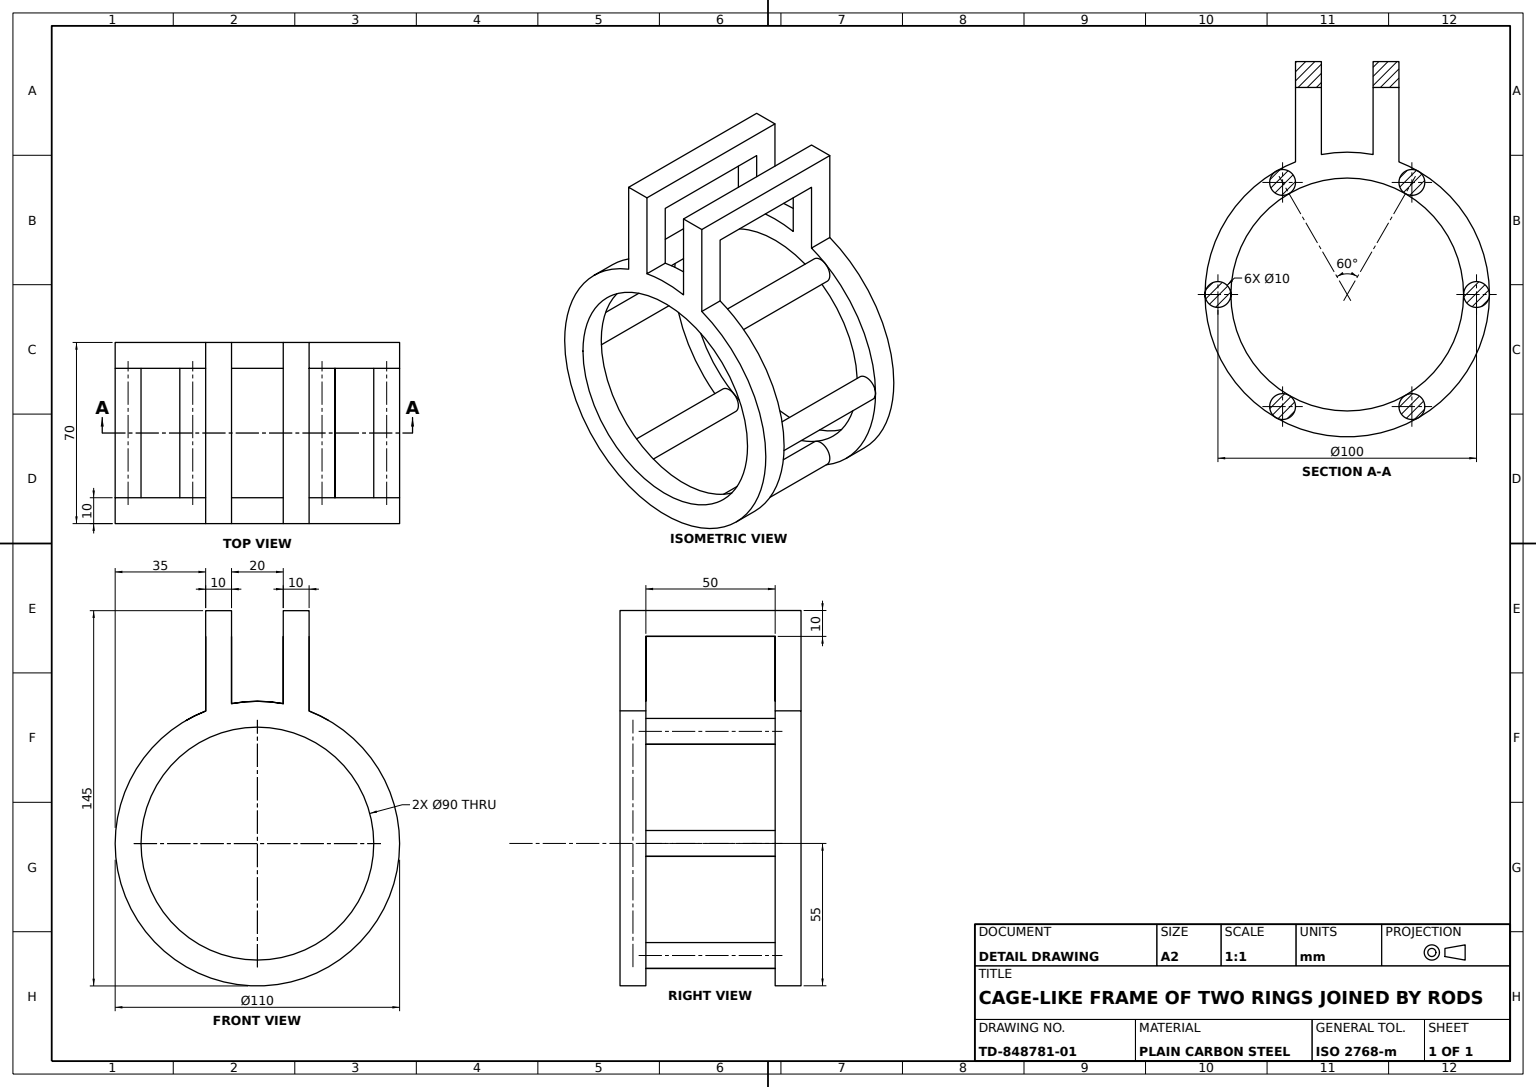
SolidWorks part; units mm, degrees
material "Plain Carbon Steel"
ref_plane "Front Plane" through (0, 0, 0) normal (0, 0, 1) x (1, 0, 0)
ref_plane "Top Plane" through (0, 0, 0) normal (0, 1, 0) x (1, 0, 0)
ref_plane "Right Plane" through (0, 0, 0) normal (1, 0, 0) x (0, 0, -1)
sketch "Front Ring Profile Ø110" plane through (0, 0, 0) normal (0, 0, 1) x (1, 0, 0)
  circle A0 centre (0, 0) radius 55
  dimension "D1" = 110
extrude "Front Ring Disc" add sketch "Front Ring Profile Ø110" against normal blind 10
ref_plane "Plane1" through (0, 0, -70) normal (0, 0, 1) x (1, 0, 0)
sketch "Rear Ring Profile" plane through (0, 0, -70) normal (0, 0, 1) x (1, 0, 0)
  circle A0 centre (0, 0) radius 55 construction
  circle A1 centre (0, 0) radius 55
extrude "Rear Ring Disc" add sketch "Rear Ring Profile" along normal blind 10 separate body
sketch "Ring Bore Ø90 Profile" plane through (0, 0, 0) normal (0, 0, 1) x (1, 0, 0)
  circle A0 centre (0, 0) radius 45
  dimension "D1" = 90
extrude "Ring Bore Ø90" cut sketch "Ring Bore Ø90 Profile" against normal through all
ref_plane "Plane2" through (20, 0, 0) normal (1, 0, 0) x (0, 0, -1)
sketch "Front Clamp Bracket Profile" plane through (20, 0, 0) normal (1, 0, 0) x (0, 0, -1)
  line L0 (0, 45) -> (0, 90)
  line L1 (0, 55) -> (0, -55) construction
  line L2 (0, 90) -> (70, 90)
  line L3 (70, 90) -> (70, 45)
  line L4 (70, -55) -> (70, 55) construction
  line L5 (0, 45) -> (10, 45)
  line L6 (10, -55) -> (10, 55) construction
  line L7 (10, 45) -> (10, 80)
  line L8 (10, 80) -> (60, 80)
  line L9 (60, 80) -> (60, 45)
  line L10 (60, 55) -> (60, -55) construction
  line L11 (60, 45) -> (70, 45)
  dimension "D1" = 90
  dimension "D2" = 50
  dimension "D3" = 10
  dimension "D4" = 45
  dimension "D5" = 70
extrude "Front Clamp Bracket" add sketch "Front Clamp Bracket Profile" against normal blind 10
ref_plane "Plane3" through (-20, 0, 0) normal (1, 0, 0) x (0, 0, -1)
sketch "Rear Clamp Bracket Profile" plane through (-20, 0, 0) normal (1, 0, 0) x (0, 0, -1)
  line L0 (10, 80) -> (60, 80) construction
  line L1 (60, 80) -> (60, 51.2348) construction
  line L2 (60, 51.2348) -> (70, 51.2348) construction
  line L3 (10, 51.2348) -> (10, 80) construction
  line L4 (0, 51.2348) -> (10, 51.2348) construction
  line L5 (70, 51.2348) -> (70, 90) construction
  line L6 (0, 90) -> (0, 51.2348) construction
  line L7 (70, 90) -> (0, 90) construction
  line L8 (10, 80) -> (60, 80)
  line L9 (60, 80) -> (60, 51.2348)
  line L10 (60, 51.2348) -> (70, 51.2348)
  line L11 (10, 51.2348) -> (10, 80)
  line L12 (0, 51.2348) -> (10, 51.2348)
  line L13 (70, 51.2348) -> (70, 90)
  line L14 (0, 90) -> (0, 51.2348)
  line L15 (70, 90) -> (0, 90)
extrude "Rear Clamp Bracket" add sketch "Rear Clamp Bracket Profile" along normal blind 10
sketch "Cage Rods 6xØ10 Profile" plane through (0, 0, -10) normal (0, 0, -1) x (-1, 0, 0)
  circle A0 centre (50, 0) radius 5
  arc A1 (-20, 51.2348) -> (20, 51.2348) centre (0, 0) ccw construction
  circle A3 centre (25, -43.3013) radius 5
  circle A4 centre (-25, -43.3013) radius 5
  circle A5 centre (-50, 0) radius 5
  circle A6 centre (-25, 43.3013) radius 5
  circle A7 centre (25, 43.3013) radius 5
  dimension "D1" = 10
  dimension "D2" = 6
extrude "Cage Rods 6xØ10" add sketch "Cage Rods 6xØ10 Profile" along normal blind 50
